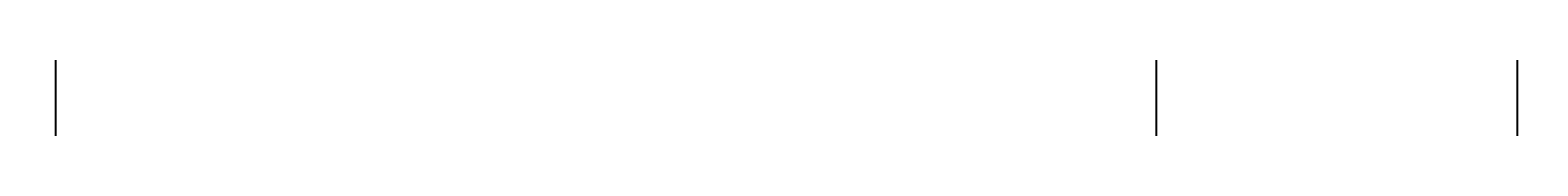
# Model space of a CAD drawing. Units: inches. Extents: x 35362 to 73946, y 43607 to 67532.
# Tile 81 of 134: x 50119 to 51337, y 47497 to 47543. Entities that reach past the tile are written whole.
import ezdxf

# ---------------------------------------------------------------- set-up
doc = ezdxf.new("R2010")
doc.units = ezdxf.units.IN
doc.header["$MEASUREMENT"] = 0
doc.layers.add('A-ANNO-DIMS', color=2, linetype='Continuous', lineweight=18)
doc.styles.get("Standard").update_dxf_attribs({"font": 'arial.ttf'})
doc.dimstyles.get("Standard").update_dxf_attribs({"dimtxt": 0.18, "dimasz": 0.18, "dimexe": 0.18, "dimexo": 0.0625, "dimgap": 0.09, "dimtad": 0, "dimtih": 1, "dimtoh": 1, "dimdec": 4, "dimzin": 0, "dimdsep": 46, "dimtxsty": 'Standard', "dimcen": 0.09, "dimadec": 0, "dimazin": 0, "dimtfac": 1, "dimtdec": 4, "dimtofl": 0, "dimtmove": 0, "dimatfit": 3, "dimfxl": 1, "dimtolj": 1, "dimtzin": 0, "dimarcsym": 0})

# ---------------------------------------------------------------- blocks, each defined once
blk = doc.blocks.new('*D11')
at = {"layer": 'A-ANNO-DIMS', "color": 0, "lineweight": -2, "transparency": 16777216}
for p, q in [((47978.7, 56028.8), (47978.7, 43606.7)), ((53109.8, 56028.8), (53109.8, 43606.7)), ((47978.8, 43606.9), (50543.9, 43606.9)), ((53109.6, 43606.9), (50544.6, 43606.9))]:
    blk.add_line(p, q, dxfattribs=at)
at = {"layer": 'A-ANNO-DIMS', "color": 0, "transparency": 16777216}
for points in [[(47978.8, 43606.9), (47978.8, 43606.8), (47978.7, 43606.9)], [(53109.6, 43606.9), (53109.6, 43606.8), (53109.8, 43606.9)]]:
    blk.add_solid(points, dxfattribs=at)
at = {"layer": 'Defpoints', "color": 0, "transparency": 16777216}
for p in [(47978.7, 56028.8), (53109.8, 56028.8), (53109.8, 43606.9)]:
    blk.add_point(p, dxfattribs=at)
at = {"layer": 'A-ANNO-DIMS', "color": 0, "transparency": 16777216, "insert": (50544.2, 43606.9), "char_height": 0.18, "attachment_point": 5}
blk.add_mtext('\\A1;5131', dxfattribs=at)
blk = doc.blocks.new('*D13')
at = {"layer": 'A-ANNO-DIMS', "color": 0, "lineweight": -2, "transparency": 16777216}
for p, q in [((48373.5, 51694), (48373.5, 43606.7)), ((51029, 51694), (51029, 43606.7)), ((48373.7, 43606.9), (49700.8, 43606.9)), ((51028.9, 43606.9), (49701.7, 43606.9))]:
    blk.add_line(p, q, dxfattribs=at)
at = {"layer": 'A-ANNO-DIMS', "color": 0, "transparency": 16777216}
for points in [[(48373.7, 43606.9), (48373.7, 43606.8), (48373.5, 43606.9)], [(51028.9, 43606.9), (51028.9, 43606.8), (51029, 43606.9)]]:
    blk.add_solid(points, dxfattribs=at)
at = {"layer": 'Defpoints', "color": 0, "transparency": 16777216}
for p in [(48373.5, 51694.1), (51029, 51694.1), (51029, 43606.9)]:
    blk.add_point(p, dxfattribs=at)
at = {"layer": 'A-ANNO-DIMS', "color": 0, "transparency": 16777216, "insert": (49701.3, 43606.9), "char_height": 0.18, "attachment_point": 5}
blk.add_mtext('\\A1;2655.6', dxfattribs=at)
blk = doc.blocks.new('*D17')
at = {"layer": 'A-ANNO-DIMS', "color": 0, "lineweight": -2, "transparency": 16777216}
for p, q in [((49923.3, 61293.2), (49923.3, 43606.7)), ((51913.9, 61293.2), (51913.9, 43606.7)), ((49923.5, 43606.9), (50918.2, 43606.9)), ((51913.8, 43606.9), (50919.1, 43606.9))]:
    blk.add_line(p, q, dxfattribs=at)
at = {"layer": 'A-ANNO-DIMS', "color": 0, "transparency": 16777216}
for points in [[(49923.5, 43606.9), (49923.5, 43606.8), (49923.3, 43606.9)], [(51913.8, 43606.9), (51913.8, 43606.8), (51913.9, 43606.9)]]:
    blk.add_solid(points, dxfattribs=at)
at = {"layer": 'Defpoints', "color": 0, "transparency": 16777216}
for p in [(49923.3, 61293.3), (51913.9, 61293.3), (51913.9, 43606.9)]:
    blk.add_point(p, dxfattribs=at)
at = {"layer": 'A-ANNO-DIMS', "color": 0, "transparency": 16777216, "insert": (50918.6, 43606.9), "char_height": 0.18, "attachment_point": 5}
blk.add_mtext('\\A1;1990.6', dxfattribs=at)
blk = doc.blocks.new('*D43')
at = {"layer": 'A-ANNO-DIMS', "color": 0, "lineweight": -2, "transparency": 16777216}
for p, q in [((62004.7, 47625.2), (35361.8, 47625.2)), ((35361.9, 47625), (35361.9, 47416.9)), ((35361.9, 47208.4), (35361.9, 47416.5)), ((62004.7, 47208.2), (35361.8, 47208.2))]:
    blk.add_line(p, q, dxfattribs=at)
at = {"layer": 'A-ANNO-DIMS', "color": 0, "transparency": 16777216}
for points in [[(35361.9, 47625), (35362, 47625), (35361.9, 47625.2)], [(35361.9, 47208.4), (35362, 47208.4), (35361.9, 47208.2)]]:
    blk.add_solid(points, dxfattribs=at)
at = {"layer": 'Defpoints', "color": 0, "transparency": 16777216}
for p in [(62004.7, 47625.2), (35361.9, 47208.2), (62004.7, 47208.2)]:
    blk.add_point(p, dxfattribs=at)
at = {"layer": 'A-ANNO-DIMS', "color": 0, "transparency": 16777216, "insert": (35361.9, 47416.7), "char_height": 0.18, "attachment_point": 5}
blk.add_mtext('\\A1;416.9', dxfattribs=at)
blk = doc.blocks.new('*D67')
at = {"layer": 'A-ANNO-DIMS', "color": 0, "lineweight": -2, "transparency": 16777216}
for p, q in [((56873.5, 53351.5), (35361.8, 53351.5)), ((35361.9, 53351.3), (35361.9, 49400.9)), ((35361.9, 45450.1), (35361.9, 49400.5)), ((53793.6, 45449.9), (35361.8, 45449.9))]:
    blk.add_line(p, q, dxfattribs=at)
at = {"layer": 'A-ANNO-DIMS', "color": 0, "transparency": 16777216}
for points in [[(35361.9, 53351.3), (35362, 53351.3), (35361.9, 53351.5)], [(35361.9, 45450.1), (35362, 45450.1), (35361.9, 45449.9)]]:
    blk.add_solid(points, dxfattribs=at)
at = {"layer": 'Defpoints', "color": 0, "transparency": 16777216}
for p in [(35361.9, 53351.5), (56873.6, 53351.5), (53793.6, 45449.9)]:
    blk.add_point(p, dxfattribs=at)
at = {"layer": 'A-ANNO-DIMS', "color": 0, "transparency": 16777216, "insert": (35361.9, 49400.7), "char_height": 0.18, "attachment_point": 5}
blk.add_mtext('\\A1;7901.6', dxfattribs=at)
blk = doc.blocks.new('*D107')
at = {"layer": 'A-ANNO-DIMS', "color": 0, "lineweight": -2, "transparency": 16777216}
for p, q in [((50139.6, 59850), (50139.6, 43606.7)), ((51320.8, 59850), (51320.8, 43606.7)), ((50139.7, 43606.9), (50729.7, 43606.9)), ((51320.6, 43606.9), (50730.6, 43606.9))]:
    blk.add_line(p, q, dxfattribs=at)
at = {"layer": 'A-ANNO-DIMS', "color": 0, "transparency": 16777216}
for points in [[(50139.7, 43606.9), (50139.7, 43606.8), (50139.6, 43606.9)], [(51320.6, 43606.9), (51320.6, 43606.8), (51320.8, 43606.9)]]:
    blk.add_solid(points, dxfattribs=at)
at = {"layer": 'Defpoints', "color": 0, "transparency": 16777216}
for p in [(50139.6, 59850.1), (51320.8, 59850.1), (51320.8, 43606.9)]:
    blk.add_point(p, dxfattribs=at)
at = {"layer": 'A-ANNO-DIMS', "color": 0, "transparency": 16777216, "insert": (50730.2, 43606.9), "char_height": 0.18, "attachment_point": 5}
blk.add_mtext('\\A1;1181.3', dxfattribs=at)

msp = doc.modelspace()

# ---------------------------------------------------------------- dimensions: what is measured, and where the dimension line sits
at = {"layer": 'A-ANNO-DIMS'}
for base, p1, p2, override, picture, middle in [((51913.931, 43606.859), (49923.307, 61293.286), (51913.931, 61293.286), {"dimdec": 1, "dimlfac": 1, "dimrnd": 0, "dimzin": 0, "dimdsep": 46, "dimlunit": 2}, '*D17', (50918.619, 43606.859)), ((51320.8133, 43606.859), (50139.5627, 59850.0769), (51320.8133, 59850.0769), {"dimdec": 1, "dimlfac": 1, "dimrnd": 0, "dimzin": 0, "dimdsep": 46, "dimlunit": 2}, '*D107', (50730.188, 43606.859)), ((53109.76, 43606.859), (47978.665, 56028.836), (53109.76, 56028.836), {"dimdec": 0, "dimlfac": 1, "dimrnd": 0, "dimzin": 0, "dimdsep": 46, "dimlunit": 2}, '*D11', (50544.212, 43606.859)), ((51029.043, 43606.859), (48373.492, 51694.087), (51029.043, 51694.087), {"dimdec": 1, "dimlfac": 1, "dimrnd": 0, "dimzin": 0, "dimdsep": 46, "dimlunit": 2}, '*D13', (49701.267, 43606.859))]:
    dim = msp.add_linear_dim(base=base, p1=p1, p2=p2, dimstyle='Standard', override=override, dxfattribs=at)
    dim.commit()
    dim.dimension.update_dxf_attribs({"geometry": picture, "text_midpoint": middle})
for base, p1, p2, picture, middle in [((35361.949, 53351.529), (53793.638, 45449.894), (56873.602, 53351.529), '*D67', (35361.949, 49400.712)), ((35361.949, 47208.25), (62004.728, 47625.181), (62004.728, 47208.25), '*D43', (35361.949, 47416.715))]:
    dim = msp.add_linear_dim(base=base, p1=p1, p2=p2, angle=90, dimstyle='Standard', override={"dimdec": 1, "dimlfac": 1, "dimrnd": 0, "dimzin": 0, "dimdsep": 46, "dimlunit": 2}, dxfattribs=at)
    dim.commit()
    dim.dimension.update_dxf_attribs({"geometry": picture, "text_midpoint": middle})

doc.saveas('drawing.dxf')
